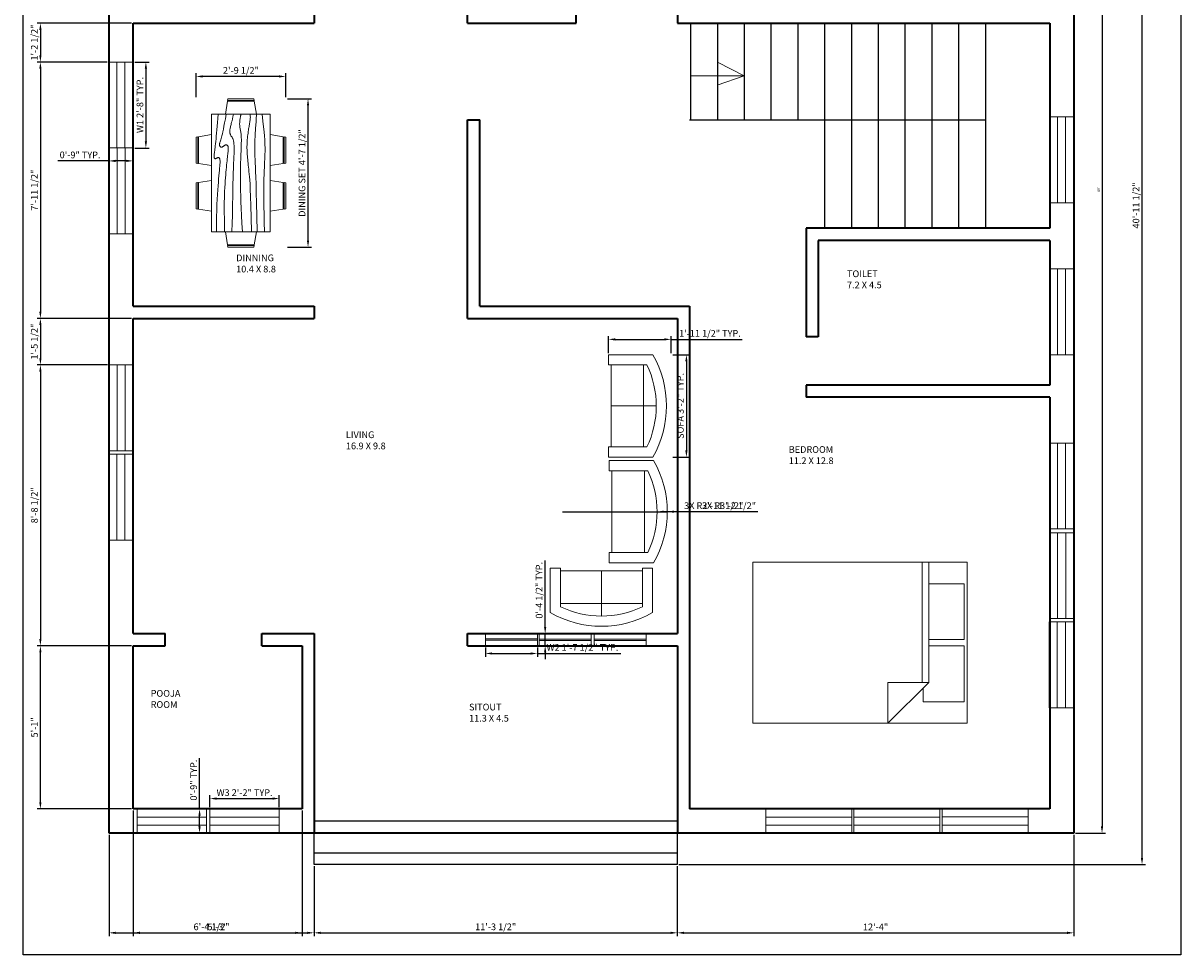
# Model space of a CAD drawing. Units: inches. Extents: x 185 to 617, y 27 to 601.
# Tile 1 of 2: x 185 to 617, y 27 to 374. Entities that reach past the tile are written whole.
import ezdxf

# ---------------------------------------------------------------- set-up
doc = ezdxf.new("R2010")
doc.units = ezdxf.units.IN
for name, color, linetype, lineweight in [('A-ANNO-DIMS', 2, 'Continuous', 18), ('A-ANNO-SYMB', 3, 'Continuous', 18), ('A-ANNO-TTLB', 7, 'Continuous', 25), ('A-AREA-IDEN', 7, 'Continuous', 18), ('A-FLOR-STRS', 7, 'Continuous', 25), ('A-FURN', 8, 'Continuous', 18), ('A-GLAZ', 4, 'Continuous', 18), ('A-WALL', 7, 'Continuous', 35)]:
    doc.layers.add(name, color=color, linetype=linetype, lineweight=lineweight)
doc.styles.get("Standard").update_dxf_attribs({"font": 'arial.ttf'})
doc.dimstyles.new('ISO-25', dxfattribs={"dimtxt": 2.5, "dimasz": 2.5, "dimexe": 1.25, "dimexo": 0.625, "dimtad": 1, "dimtxsty": 'Standard', "dimcen": 2.5, "dimadec": 0, "dimazin": 0, "dimtfac": 1, "dimtmove": 0, "dimatfit": 3, "dimfxl": 1, "dimarcsym": 0})

# ---------------------------------------------------------------- blocks, each defined once
blk = doc.blocks.new('Sofa - Roundback Loveseat 5 ft.')
for p, q in [((0, -32.44198), (0, -5.99998)), ((-24, -33.99998), (-24, -11.46958)), ((-23.9998, -13.38178), (23.99986, -13.38178)), ((24.00004, -33.99998), (24.00004, -11.46958)), ((-24, -32.44198), (24.00004, -32.44198))]:
    blk.add_line(p, q)
for points in [[(-24, -33.99998), (-30, -33.99998), (-30, -7.99998)], [(30.00004, -7.99998), (30.00004, -33.99998), (24.00004, -33.99998)]]:
    blk.add_lwpolyline(points)
for centre, radius, start, end in [((0, -60.24998), 60.24998, 60.13715, 119.8628), ((0, -61.38438), 55.38444, 64.32083, 115.6792)]:
    blk.add_arc(centre, radius, start, end)
blk = doc.blocks.new('Dining Set - 36 x 72 in.')
for p, q in [((-22.2343, 26.00059), (-23.4847, 17.99762)), ((-22.2304, 26), (-5.7608, 26)), ((-22, 27.5), (-22.1562, 26.50042)), ((-5.8416, 26.5), (-22.1534, 26.5)), ((-22, 27.5), (-6, 27.5)), ((-5.8437, 26.49966), (-6, 27.5)), ((-4.5152, 17.99762), (-5.7655, 25.99926)), ((5.7657, 26.00059), (4.5153, 17.99762)), ((5.7696, 26), (22.2392, 26)), ((6, 27.5), (5.8438, 26.50042)), ((22.1584, 26.5), (5.8466, 26.5)), ((6, 27.5), (22, 27.5)), ((22.1563, 26.49966), (22, 27.5)), ((23.4848, 17.99762), (22.2345, 25.99926)), ((36, 18), (-36, 18)), ((-36, 18), (-36, -18)), ((36, -18), (36, 18)), ((-45.5, 8), (-44.5004, 8.15617)), ((-45.5, 8), (-45.5, -8)), ((-44.5, -8.15843), (-44.5, 8.15338)), ((-44.0006, 8.23428), (-35.9976, 9.48474)), ((-44, 8.23041), (-44, -8.23915)), ((44.0006, 8.23428), (35.9976, 9.48474)), ((44, 8.23041), (44, -8.23915)), ((44.5, -8.15843), (44.5, 8.15338)), ((45.5, 8), (44.5005, 8.15617)), ((45.5, 8), (45.5, -8)), ((-44.4997, -8.15631), (-45.5, -8)), ((-35.9976, -9.48476), (-43.9993, -8.2345)), ((35.9976, -9.48476), (43.9993, -8.2345)), ((44.4997, -8.15631), (45.5, -8)), ((-36, -18), (36, -18)), ((-22.2343, -26.0006), (-23.4847, -17.99762)), ((-4.5152, -17.99762), (-5.7655, -25.99928)), ((5.7657, -26.0006), (4.5153, -17.99762)), ((23.4848, -17.99762), (22.2345, -25.99928)), ((-22.2304, -26), (-5.7608, -26)), ((-22, -27.5), (-22.1562, -26.50044)), ((-5.8416, -26.5), (-22.1534, -26.5)), ((-22, -27.5), (-6, -27.5)), ((-5.8437, -26.49967), (-6, -27.5)), ((5.7696, -26), (22.2392, -26)), ((6, -27.5), (5.8438, -26.50044)), ((22.1584, -26.5), (5.8466, -26.5)), ((6, -27.5), (22, -27.5)), ((22.1563, -26.49967), (22, -27.5))]:
    blk.add_line(p, q)
for points in [[(-36, 15), (-31.1772, 14.97754), (-26.8079, 14.91406), (-22.8538, 14.81543), (-19.276, 14.6875), (-16.0362, 14.53613), (-13.0957, 14.36718), (-10.4159, 14.18652), (-7.9583, 14), (-5.6904, 13.81315), (-3.6035, 13.63021), (-1.6954, 13.45508), (0.0365, 13.29166), (1.5945, 13.14388), (2.9811, 13.01562), (4.1988, 12.9108), (5.25, 12.83333), (6.1393, 12.78613), (6.8802, 12.76823), (7.4883, 12.77767), (7.9792, 12.8125), (8.3685, 12.87077), (8.6719, 12.95052), (8.9049, 13.0498), (9.0833, 13.16666), (9.2205, 13.29899), (9.3216, 13.44401), (9.3895, 13.59879), (9.4271, 13.76041), (9.4373, 13.92594), (9.4232, 14.09245), (9.3875, 14.257), (9.3333, 14.41666), (9.2638, 14.56917), (9.1836, 14.71484), (9.0975, 14.85465), (9.0104, 14.98958), (8.9272, 15.1206), (8.8529, 15.2487), (8.7922, 15.37483), (8.75, 15.5), (8.7305, 15.62467), (8.7344, 15.74739), (8.7617, 15.86621), (8.8125, 15.97916), (8.8867, 16.08431), (8.9844, 16.17968), (9.1055, 16.26334), (9.25, 16.33333), (9.4189, 16.38802), (9.6172, 16.42708), (9.8506, 16.45052), (10.125, 16.45833), (10.4463, 16.45052), (10.8203, 16.42708), (11.2529, 16.38802), (11.75, 16.33333), (12.3184, 16.26318), (12.9694, 16.17838), (13.7151, 16.07991), (14.5677, 15.96875), (15.5395, 15.84586), (16.6426, 15.71224), (17.8893, 15.56884), (19.2917, 15.41666), (20.859, 15.25667), (22.5879, 15.08984), (24.4721, 14.91715), (26.5052, 14.73958), (28.6809, 14.5581), (30.9929, 14.3737), (33.4347, 14.18733), (36, 14)], [(-36, 10), (-28.9766, 10.14274), (-23.1725, 10.20442), (-18.4241, 10.19775), (-14.5677, 10.13541), (-11.4399, 10.03011), (-8.877, 9.89453), (-6.7154, 9.74137), (-4.7917, 9.58333), (-2.9698, 9.43082), (-1.2246, 9.28515), (0.4415, 9.14534), (2.026, 9.01041), (3.5266, 8.87939), (4.9408, 8.7513), (6.266, 8.62516), (7.5, 8.5), (8.6411, 8.37549), (9.6914, 8.2539), (10.6538, 8.13818), (11.5312, 8.03125), (12.3267, 7.93603), (13.043, 7.85547), (13.6831, 7.79248), (14.25, 7.75), (14.7471, 7.7303), (15.1797, 7.73307), (15.5537, 7.75732), (15.875, 7.80208), (16.1494, 7.86637), (16.3828, 7.94922), (16.5811, 8.04964), (16.75, 8.16666), (16.8944, 8.29915), (17.0143, 8.44531), (17.1089, 8.60319), (17.1771, 8.77083), (17.218, 8.94629), (17.2305, 9.1276), (17.2137, 9.31282), (17.1667, 9.5), (17.0895, 9.6875), (16.987, 9.875), (16.8649, 10.0625), (16.7292, 10.25), (16.5856, 10.4375), (16.4401, 10.625), (16.2985, 10.8125), (16.1667, 11), (16.05, 11.18733), (15.9518, 11.3737), (15.8752, 11.5581), (15.8229, 11.73958), (15.798, 11.91715), (15.8034, 12.08984), (15.842, 12.25667), (15.9167, 12.41666), (16.0295, 12.56836), (16.1784, 12.70833), (16.3605, 12.83268), (16.5729, 12.9375), (16.8127, 13.01888), (17.0768, 13.07291), (17.3625, 13.0957), (17.6667, 13.08333), (17.9894, 13.03312), (18.3418, 12.94726), (18.7382, 12.82918), (19.1927, 12.68229), (19.7195, 12.51001), (20.3327, 12.31575), (21.0465, 12.10294), (21.875, 11.875), (22.8357, 11.63354), (23.959, 11.37304), (25.2786, 11.08618), (26.8282, 10.76562), (28.6414, 10.40405), (30.752, 9.99414), (33.1936, 9.52856), (36, 9)], [(-36, 5.5), (-30.7157, 5.3348), (-26.069, 5.20963), (-21.9946, 5.11767), (-18.4271, 5.05208), (-15.3009, 5.00602), (-12.5508, 4.97265), (-10.1112, 4.94515), (-7.9167, 4.91666), (-5.909, 4.88167), (-4.0586, 4.83984), (-2.3429, 4.79215), (-0.7396, 4.73958), (0.7739, 4.6831), (2.22, 4.6237), (3.6213, 4.56233), (5, 4.5), (6.373, 4.43782), (7.7344, 4.3776), (9.0723, 4.32129), (10.375, 4.27083), (11.6309, 4.22819), (12.8281, 4.19531), (13.9551, 4.17415), (15, 4.16666), (15.954, 4.17448), (16.819, 4.19791), (17.6001, 4.23698), (18.3021, 4.29166), (18.9299, 4.36198), (19.4883, 4.44791), (19.9823, 4.54948), (20.4167, 4.66666), (20.7969, 4.79899), (21.1302, 4.94401), (21.4245, 5.09879), (21.6875, 5.26041), (21.9271, 5.42594), (22.1511, 5.59245), (22.3672, 5.757), (22.5834, 5.91666), (22.8065, 6.06868), (23.0404, 6.21093), (23.2879, 6.34147), (23.5521, 6.45833), (23.8358, 6.55957), (24.142, 6.64323), (24.4735, 6.70735), (24.8334, 6.75), (25.2235, 6.76969), (25.642, 6.76692), (26.0858, 6.74267), (26.5521, 6.69791), (27.0379, 6.63362), (27.5404, 6.55078), (28.0565, 6.45036), (28.5834, 6.33333), (29.1242, 6.19987), (29.7071, 6.04687), (30.3661, 5.87044), (31.1354, 5.66666), (32.0493, 5.43164), (33.142, 5.16146), (34.4475, 4.85221), (36, 4.5)], [(-36, -1), (-30.7915, -0.6591), (-26.0195, -0.38216), (-21.6519, -0.16284), (-17.6563, 0.00521), (-14.0005, 0.12833), (-10.6523, 0.21289), (-7.5796, 0.26522), (-4.75, 0.29166), (-2.134, 0.29793), (0.2878, 0.28711), (2.5317, 0.26163), (4.6146, 0.22396), (6.5529, 0.17651), (8.3633, 0.12174), (10.0623, 0.06209), (11.6667, 0), (13.1899, -0.06201), (14.6341, -0.1211), (15.9982, -0.17432), (17.2813, -0.21875), (18.4823, -0.25147), (19.6003, -0.26953), (20.6343, -0.27002), (21.5834, -0.25), (22.4481, -0.20768), (23.2357, -0.14584), (23.9549, -0.06836), (24.6146, 0.02083), (25.2235, 0.11784), (25.7904, 0.21875), (26.3241, 0.31966), (26.8334, 0.41666), (27.3265, 0.50618), (27.8099, 0.58593), (28.2894, 0.65397), (28.7709, 0.70833), (29.2601, 0.74707), (29.763, 0.76823), (30.2855, 0.76985), (30.8334, 0.75), (31.4088, 0.70784), (31.9994, 0.64713), (32.589, 0.57275), (33.1615, 0.48958), (33.7008, 0.4025), (34.1908, 0.3164), (34.6153, 0.23616), (34.9584, 0.16666), (35.2099, 0.11165), (35.3848, 0.07031), (35.504, 0.04069), (35.5886, 0.02083), (35.6594, 0.00879), (35.7377, 0.0026), (35.8442, 0.00032), (36, 0)], [(-36, -6.5), (-27.1843, -6.31267), (-20.084, -6.1263), (-14.469, -5.9419), (-10.1094, -5.76042), (-6.7752, -5.58285), (-4.2363, -5.41016), (-2.2629, -5.24333), (-0.625, -5.08334), (0.8708, -4.93099), (2.2715, -4.78646), (3.5872, -4.64974), (4.8281, -4.52084), (6.0046, -4.39974), (7.127, -4.28646), (8.2053, -4.18099), (9.25, -4.08334), (10.2705, -3.99382), (11.2734, -3.91407), (12.2647, -3.84603), (13.25, -3.79167), (14.2354, -3.75293), (15.2266, -3.73177), (16.2295, -3.73015), (17.25, -3.75), (18.2912, -3.79248), (19.3451, -3.85547), (20.4009, -3.93604), (21.4479, -4.03125), (22.4754, -4.13819), (23.4727, -4.25391), (24.4289, -4.37549), (25.3334, -4.5), (26.1785, -4.62492), (26.9694, -4.74935), (27.7145, -4.87281), (28.4219, -4.99479), (29.1, -5.11483), (29.7572, -5.23242), (30.4016, -5.34709), (31.0417, -5.45834), (31.6837, -5.56437), (32.3262, -5.65821), (32.9658, -5.73153), (33.599, -5.77604), (34.2224, -5.78345), (34.8327, -5.74545), (35.4264, -5.65373), (36, -5.5)], [(-36, -10), (-26.4022, -9.81299), (-18.4675, -9.62891), (-11.9839, -9.45069), (-6.7396, -9.28125), (-2.5226, -9.12354), (0.8789, -8.98047), (3.6769, -8.85498), (6.0833, -8.75), (8.2767, -8.66765), (10.3021, -8.60677), (12.1712, -8.56543), (13.8958, -8.54167), (15.4876, -8.53353), (16.9583, -8.53907), (18.3197, -8.55632), (19.5834, -8.58334), (20.7616, -8.61841), (21.8685, -8.66081), (22.9188, -8.71004), (23.9271, -8.76563), (24.9081, -8.82707), (25.8763, -8.89388), (26.8465, -8.96558), (27.8334, -9.04167), (28.8474, -9.12118), (29.8828, -9.20117), (30.93, -9.27824), (31.9792, -9.34896), (33.0205, -9.40991), (34.0443, -9.45768), (35.0407, -9.48885), (36, -9.5)], [(-36, -14.5), (-30.0881, -14.33513), (-25.0332, -14.21224), (-20.7312, -14.12647), (-17.0781, -14.07292), (-13.97, -14.04671), (-11.3027, -14.04297), (-8.9724, -14.05681), (-6.875, -14.08334), (-4.9224, -14.11833), (-3.0905, -14.16016), (-1.3709, -14.20785), (0.2448, -14.26042), (1.7647, -14.3169), (3.1973, -14.3763), (4.5507, -14.43767), (5.8333, -14.5), (7.0554, -14.5621), (8.235, -14.62175), (9.3922, -14.67652), (10.5469, -14.72396), (11.7192, -14.76164), (12.929, -14.78711), (14.1965, -14.79794), (15.5417, -14.79167), (16.9933, -14.76424), (18.6152, -14.70508), (20.4804, -14.60197), (22.6615, -14.44271), (25.2312, -14.21509), (28.2624, -13.9069), (31.8277, -13.50594), (36, -13)]]:
    blk.add_lwpolyline(points)
blk = doc.blocks.new('Bed - Queen')
for p, q in [((0, -80.00003), (0, 0)), ((0, 0), (59.99999, 0)), ((59.99999, 0), (59.99999, -80.00003)), ((7.99999, -1.2), (28.79998, -1.2)), ((7.99999, -14.4), (7.99999, -1.2)), ((28.79998, -1.2), (28.79998, -14.4)), ((31.19999, -1.2), (51.99999, -1.2)), ((31.19999, -14.4), (31.19999, -1.2)), ((51.99999, -1.2), (51.99999, -16.4)), ((0, -14.4), (44.8, -14.4)), ((44.8, -16.8), (0, -16.8)), ((59.99999, -29.6), (44.8, -14.4)), ((44.8, -14.4), (44.8, -29.6)), ((51.99999, -16.4), (46.79936, -16.4)), ((44.8, -29.6), (59.99999, -29.6)), ((59.99999, -80.00003), (0, -80.00003))]:
    blk.add_line(p, q)
blk = doc.blocks.new('*D7')
at = {"layer": 'A-ANNO-DIMS', "color": 0, "lineweight": -2, "transparency": 16777216}
for p, q in [((577.73, 552.31), (588.89, 552.31)), ((587.64, 549.81), (587.64, 74.81)), ((577.73, 72.31), (588.89, 72.31))]:
    blk.add_line(p, q, dxfattribs=at)
at = {"layer": 'A-ANNO-DIMS', "color": 0, "transparency": 16777216}
for points in [[(587.22, 549.81), (588.05, 549.81), (587.64, 552.31)], [(587.22, 74.81), (588.05, 74.81), (587.64, 72.31)]]:
    blk.add_solid(points, dxfattribs=at)
at = {"layer": 'Defpoints', "color": 0, "transparency": 16777216}
for p in [(577.11, 552.31), (577.11, 72.31), (587.64, 72.31)]:
    blk.add_point(p, dxfattribs=at)
at = {"layer": 'A-ANNO-DIMS', "color": 0, "transparency": 16777216, "insert": (586.5, 312.31), "char_height": 1, "attachment_point": 5, "rotation": 90}
blk.add_mtext("40'", dxfattribs=at)
blk = doc.blocks.new('WIN-32IN-EXT')
for p, q in [((0, 0), (0, 32.06)), ((0, 32.06), (9, 32.06)), ((3, 32.06), (3, 0)), ((6, 0), (6, 32.06)), ((9, 32.06), (9, 0)), ((9, 0), (0, 0))]:
    blk.add_line(p, q)
blk = doc.blocks.new('WIN-19IN-SITOUT')
for p, q in [((0, 0), (0, 4.5)), ((0, 4.5), (19.38, 4.5)), ((19.38, 4.5), (19.38, 0)), ((0, 2.5), (19.38, 2.5)), ((19.38, 2), (0, 2)), ((19.38, 0), (0, 0))]:
    blk.add_line(p, q)
blk = doc.blocks.new('WIN-26IN-EXT')
for p, q in [((0, 0), (0, 9)), ((0, 9), (25.86, 9)), ((25.86, 9), (25.86, 0)), ((25.86, 6), (0, 6)), ((0, 3), (25.86, 3)), ((25.86, 0), (0, 0))]:
    blk.add_line(p, q)
blk = doc.blocks.new('*D11')
at = {"layer": 'A-ANNO-DIMS', "color": 0, "lineweight": -2, "transparency": 16777216}
for p, q in [((226.67, 359.92), (232.11, 359.92)), ((230.86, 357.42), (230.86, 330.35)), ((226.67, 327.85), (232.11, 327.85))]:
    blk.add_line(p, q, dxfattribs=at)
at = {"layer": 'A-ANNO-DIMS', "color": 0, "transparency": 16777216}
for points in [[(230.44, 357.42), (231.27, 357.42), (230.86, 359.92)], [(230.44, 330.35), (231.27, 330.35), (230.86, 327.85)]]:
    blk.add_solid(points, dxfattribs=at)
at = {"layer": 'Defpoints', "color": 0, "transparency": 16777216}
for p in [(226.05, 359.92), (226.05, 327.85), (230.86, 327.85)]:
    blk.add_point(p, dxfattribs=at)
at = {"layer": 'A-ANNO-DIMS', "color": 0, "transparency": 16777216, "insert": (228.96, 343.88), "char_height": 2.5, "attachment_point": 5, "rotation": 90}
blk.add_mtext('W1 2\'-8" TYP.', dxfattribs=at)
blk = doc.blocks.new('*D12')
at = {"layer": 'A-ANNO-DIMS', "color": 0, "lineweight": -2, "transparency": 16777216}
for p, q in [((217.05, 327.23), (217.05, 321.79)), ((226.05, 327.23), (226.05, 321.79)), ((217.05, 323.04), (198.06, 323.04)), ((223.55, 323.04), (219.55, 323.04))]:
    blk.add_line(p, q, dxfattribs=at)
at = {"layer": 'A-ANNO-DIMS', "color": 0, "transparency": 16777216}
for points in [[(219.55, 323.46), (219.55, 322.62), (217.05, 323.04)], [(223.55, 323.46), (223.55, 322.62), (226.05, 323.04)]]:
    blk.add_solid(points, dxfattribs=at)
at = {"layer": 'Defpoints', "color": 0, "transparency": 16777216}
for p in [(217.05, 327.85), (226.05, 327.85), (217.05, 323.04)]:
    blk.add_point(p, dxfattribs=at)
at = {"layer": 'A-ANNO-DIMS', "color": 0, "transparency": 16777216, "insert": (206.3, 324.94), "char_height": 2.5, "attachment_point": 5}
blk.add_mtext('0\'-9" TYP.', dxfattribs=at)
blk = doc.blocks.new('*D13')
at = {"layer": 'A-ANNO-DIMS', "color": 0, "lineweight": -2, "transparency": 16777216}
for p, q in [((357.55, 141.6), (357.55, 138.06)), ((360.05, 139.31), (374.43, 139.31)), ((376.93, 141.6), (376.93, 138.06)), ((376.93, 139.31), (408.06, 139.31))]:
    blk.add_line(p, q, dxfattribs=at)
at = {"layer": 'A-ANNO-DIMS', "color": 0, "transparency": 16777216}
for points in [[(360.05, 139.73), (360.05, 138.9), (357.55, 139.31)], [(374.43, 139.73), (374.43, 138.9), (376.93, 139.31)]]:
    blk.add_solid(points, dxfattribs=at)
at = {"layer": 'Defpoints', "color": 0, "transparency": 16777216}
for p in [(357.55, 142.22), (376.93, 142.22), (376.93, 139.31)]:
    blk.add_point(p, dxfattribs=at)
at = {"layer": 'A-ANNO-DIMS', "color": 0, "transparency": 16777216, "insert": (393.75, 141.23), "char_height": 2.5, "attachment_point": 5}
blk.add_mtext('W2 1\'-7 1/2" TYP.', dxfattribs=at)
blk = doc.blocks.new('*D14')
at = {"layer": 'A-ANNO-DIMS', "color": 0, "lineweight": -2, "transparency": 16777216}
for p, q in [((379.84, 149.22), (379.84, 174.04)), ((377.56, 146.72), (381.09, 146.72)), ((379.84, 142.22), (379.84, 146.72)), ((377.56, 142.22), (381.09, 142.22)), ((379.84, 139.72), (379.84, 137.22))]:
    blk.add_line(p, q, dxfattribs=at)
at = {"layer": 'A-ANNO-DIMS', "color": 0, "transparency": 16777216}
for points in [[(379.42, 149.22), (380.26, 149.22), (379.84, 146.72)], [(379.42, 139.72), (380.26, 139.72), (379.84, 142.22)]]:
    blk.add_solid(points, dxfattribs=at)
at = {"layer": 'Defpoints', "color": 0, "transparency": 16777216}
for p in [(376.93, 146.72), (379.84, 146.72), (376.93, 142.22)]:
    blk.add_point(p, dxfattribs=at)
at = {"layer": 'A-ANNO-DIMS', "color": 0, "transparency": 16777216, "insert": (377.92, 162.88), "char_height": 2.5, "attachment_point": 5, "rotation": 90}
blk.add_mtext('0\'-4 1/2" TYP.', dxfattribs=at)
blk = doc.blocks.new('*D15')
at = {"layer": 'A-ANNO-DIMS', "color": 0, "lineweight": -2, "transparency": 16777216}
for p, q in [((254.75, 81.95), (254.75, 86.45)), ((280.61, 81.95), (280.61, 86.45)), ((257.25, 85.2), (278.11, 85.2))]:
    blk.add_line(p, q, dxfattribs=at)
at = {"layer": 'A-ANNO-DIMS', "color": 0, "transparency": 16777216}
for points in [[(257.25, 85.62), (257.25, 84.78), (254.75, 85.2)], [(278.11, 85.62), (278.11, 84.78), (280.61, 85.2)]]:
    blk.add_solid(points, dxfattribs=at)
at = {"layer": 'Defpoints', "color": 0, "transparency": 16777216}
for p in [(280.61, 85.2), (254.75, 81.32), (280.61, 81.32)]:
    blk.add_point(p, dxfattribs=at)
at = {"layer": 'A-ANNO-DIMS', "color": 0, "transparency": 16777216, "insert": (267.68, 87.1), "char_height": 2.5, "attachment_point": 5}
blk.add_mtext('W3 2\'-2" TYP.', dxfattribs=at)
blk = doc.blocks.new('*D16')
at = {"layer": 'A-ANNO-DIMS', "color": 0, "lineweight": -2, "transparency": 16777216}
for p, q in [((250.88, 81.32), (250.88, 100.31)), ((254.13, 81.32), (249.63, 81.32)), ((250.88, 74.82), (250.88, 78.82)), ((254.13, 72.32), (249.63, 72.32))]:
    blk.add_line(p, q, dxfattribs=at)
at = {"layer": 'A-ANNO-DIMS', "color": 0, "transparency": 16777216}
for points in [[(250.46, 78.82), (251.29, 78.82), (250.88, 81.32)], [(250.46, 74.82), (251.29, 74.82), (250.88, 72.32)]]:
    blk.add_solid(points, dxfattribs=at)
at = {"layer": 'Defpoints', "color": 0, "transparency": 16777216}
for p in [(250.88, 81.32), (254.75, 81.32), (254.75, 72.32)]:
    blk.add_point(p, dxfattribs=at)
at = {"layer": 'A-ANNO-DIMS', "color": 0, "transparency": 16777216, "insert": (248.97, 92.07), "char_height": 2.5, "attachment_point": 5, "rotation": 90}
blk.add_mtext('0\'-9" TYP.', dxfattribs=at)
blk = doc.blocks.new('*D17')
at = {"layer": 'A-ANNO-DIMS', "color": 0, "lineweight": -2, "transparency": 16777216}
for p, q in [((427.44, 250.74), (433.8, 250.74)), ((432.55, 248.24), (432.55, 215.03)), ((427.44, 212.53), (433.8, 212.53))]:
    blk.add_line(p, q, dxfattribs=at)
at = {"layer": 'A-ANNO-DIMS', "color": 0, "transparency": 16777216}
for points in [[(432.13, 248.24), (432.96, 248.24), (432.55, 250.74)], [(432.13, 215.03), (432.96, 215.03), (432.55, 212.53)]]:
    blk.add_solid(points, dxfattribs=at)
at = {"layer": 'Defpoints', "color": 0, "transparency": 16777216}
for p in [(426.82, 250.74), (426.82, 212.53), (432.55, 212.53)]:
    blk.add_point(p, dxfattribs=at)
at = {"layer": 'A-ANNO-DIMS', "color": 0, "transparency": 16777216, "insert": (430.63, 231.64), "char_height": 2.5, "attachment_point": 5, "rotation": 90}
blk.add_mtext('SOFA 3\'-2" TYP.', dxfattribs=at)
blk = doc.blocks.new('*D18')
at = {"layer": 'A-ANNO-DIMS', "color": 0, "lineweight": -2, "transparency": 16777216}
for p, q in [((403.47, 251.36), (403.47, 257.72)), ((405.97, 256.47), (424.32, 256.47)), ((426.82, 251.36), (426.82, 257.72)), ((426.82, 256.47), (453.34, 256.47))]:
    blk.add_line(p, q, dxfattribs=at)
at = {"layer": 'A-ANNO-DIMS', "color": 0, "transparency": 16777216}
for points in [[(405.97, 256.88), (405.97, 256.05), (403.47, 256.47)], [(424.32, 256.88), (424.32, 256.05), (426.82, 256.47)]]:
    blk.add_solid(points, dxfattribs=at)
at = {"layer": 'Defpoints', "color": 0, "transparency": 16777216}
for p in [(426.82, 256.47), (403.47, 250.74), (426.82, 250.74)]:
    blk.add_point(p, dxfattribs=at)
at = {"layer": 'A-ANNO-DIMS', "color": 0, "transparency": 16777216, "insert": (441.33, 258.38), "char_height": 2.5, "attachment_point": 5}
blk.add_mtext('1\'-11 1/2" TYP.', dxfattribs=at)
blk = doc.blocks.new('*D21')
at = {"layer": 'A-ANNO-DIMS', "color": 0, "lineweight": -2, "transparency": 16777216}
for p, q in [((283.68, 346.23), (292.61, 346.23)), ((291.36, 293.33), (291.36, 343.73)), ((283.68, 290.83), (292.61, 290.83))]:
    blk.add_line(p, q, dxfattribs=at)
at = {"layer": 'A-ANNO-DIMS', "color": 0, "transparency": 16777216}
for points in [[(290.95, 343.73), (291.78, 343.73), (291.36, 346.23)], [(290.95, 293.33), (291.78, 293.33), (291.36, 290.83)]]:
    blk.add_solid(points, dxfattribs=at)
at = {"layer": 'Defpoints', "color": 0, "transparency": 16777216}
for p in [(283.05, 346.23), (291.36, 346.23), (283.05, 290.83)]:
    blk.add_point(p, dxfattribs=at)
at = {"layer": 'A-ANNO-DIMS', "color": 0, "transparency": 16777216, "insert": (289.44, 318.53), "char_height": 2.5, "attachment_point": 5, "rotation": 90}
blk.add_mtext('DINING SET 4\'-7 1/2"', dxfattribs=at)
blk = doc.blocks.new('*D22')
at = {"layer": 'A-ANNO-DIMS', "color": 0, "lineweight": -2, "transparency": 16777216}
for p, q in [((249.57, 346.85), (249.57, 355.79)), ((280.55, 354.54), (252.07, 354.54)), ((283.05, 346.85), (283.05, 355.79))]:
    blk.add_line(p, q, dxfattribs=at)
at = {"layer": 'A-ANNO-DIMS', "color": 0, "transparency": 16777216}
for points in [[(252.07, 354.95), (252.07, 354.12), (249.57, 354.54)], [(280.55, 354.95), (280.55, 354.12), (283.05, 354.54)]]:
    blk.add_solid(points, dxfattribs=at)
at = {"layer": 'Defpoints', "color": 0, "transparency": 16777216}
for p in [(249.57, 354.54), (249.57, 346.23), (283.05, 346.23)]:
    blk.add_point(p, dxfattribs=at)
at = {"layer": 'A-ANNO-DIMS', "color": 0, "transparency": 16777216, "insert": (266.31, 356.46), "char_height": 2.5, "attachment_point": 5}
blk.add_mtext('2\'-9 1/2"', dxfattribs=at)
blk = doc.blocks.new('*D25')
at = {"layer": 'A-ANNO-DIMS', "color": 0, "lineweight": -2, "transparency": 16777216}
for p, q in [((577.73, 552.31), (603.81, 552.31)), ((602.56, 63.07), (602.56, 549.81)), ((429.78, 60.57), (603.81, 60.57))]:
    blk.add_line(p, q, dxfattribs=at)
at = {"layer": 'A-ANNO-DIMS', "color": 0, "transparency": 16777216}
for points in [[(602.14, 549.81), (602.97, 549.81), (602.56, 552.31)], [(602.14, 63.07), (602.97, 63.07), (602.56, 60.57)]]:
    blk.add_solid(points, dxfattribs=at)
at = {"layer": 'Defpoints', "color": 0, "transparency": 16777216}
for p in [(577.11, 552.31), (602.56, 552.31), (429.16, 60.57)]:
    blk.add_point(p, dxfattribs=at)
at = {"layer": 'A-ANNO-DIMS', "color": 0, "transparency": 16777216, "insert": (600.64, 306.44), "char_height": 2.5, "attachment_point": 5, "rotation": 90}
blk.add_mtext('40\'-11 1/2"', dxfattribs=at)
blk = doc.blocks.new('*D26')
at = {"layer": 'A-ANNO-DIMS', "color": 0, "lineweight": -2, "transparency": 16777216}
for p, q in [((226.11, 80.69), (226.11, 33.87)), ((289.11, 80.69), (289.11, 33.87)), ((228.61, 35.12), (286.61, 35.12))]:
    blk.add_line(p, q, dxfattribs=at)
at = {"layer": 'A-ANNO-DIMS', "color": 0, "transparency": 16777216}
for points in [[(228.61, 35.54), (228.61, 34.7), (226.11, 35.12)], [(286.61, 35.54), (286.61, 34.7), (289.11, 35.12)]]:
    blk.add_solid(points, dxfattribs=at)
at = {"layer": 'Defpoints', "color": 0, "transparency": 16777216}
for p in [(226.11, 81.31), (289.11, 81.31), (289.11, 35.12)]:
    blk.add_point(p, dxfattribs=at)
at = {"layer": 'A-ANNO-DIMS', "color": 0, "transparency": 16777216, "insert": (257.61, 37.02), "char_height": 2.5, "attachment_point": 5}
blk.add_mtext('5\'-3"', dxfattribs=at)
blk = doc.blocks.new('*D27')
at = {"layer": 'A-ANNO-DIMS', "color": 0, "lineweight": -2, "transparency": 16777216}
for p, q in [((225.48, 142.21), (190.25, 142.21)), ((191.5, 83.81), (191.5, 139.71)), ((225.48, 81.31), (190.25, 81.31))]:
    blk.add_line(p, q, dxfattribs=at)
at = {"layer": 'A-ANNO-DIMS', "color": 0, "transparency": 16777216}
for points in [[(191.08, 139.71), (191.91, 139.71), (191.5, 142.21)], [(191.08, 83.81), (191.91, 83.81), (191.5, 81.31)]]:
    blk.add_solid(points, dxfattribs=at)
at = {"layer": 'Defpoints', "color": 0, "transparency": 16777216}
for p in [(191.5, 142.21), (226.11, 142.21), (226.11, 81.31)]:
    blk.add_point(p, dxfattribs=at)
at = {"layer": 'A-ANNO-DIMS', "color": 0, "transparency": 16777216, "insert": (189.6, 111.76), "char_height": 2.5, "attachment_point": 5, "rotation": 90}
blk.add_mtext('5\'-1"', dxfattribs=at)
blk = doc.blocks.new('*D28')
at = {"layer": 'A-ANNO-DIMS', "color": 0, "lineweight": -2, "transparency": 16777216}
for p, q in [((217.11, 71.69), (217.11, 33.87)), ((293.59, 59.94), (293.59, 33.87)), ((219.61, 35.12), (291.09, 35.12))]:
    blk.add_line(p, q, dxfattribs=at)
at = {"layer": 'A-ANNO-DIMS', "color": 0, "transparency": 16777216}
for points in [[(219.61, 35.54), (219.61, 34.7), (217.11, 35.12)], [(291.09, 35.54), (291.09, 34.7), (293.59, 35.12)]]:
    blk.add_solid(points, dxfattribs=at)
at = {"layer": 'Defpoints', "color": 0, "transparency": 16777216}
for p in [(217.11, 72.31), (293.59, 60.57), (293.59, 35.12)]:
    blk.add_point(p, dxfattribs=at)
at = {"layer": 'A-ANNO-DIMS', "color": 0, "transparency": 16777216, "insert": (255.35, 37.04), "char_height": 2.5, "attachment_point": 5}
blk.add_mtext('6\'-4 1/2"', dxfattribs=at)
blk = doc.blocks.new('*D29')
at = {"layer": 'A-ANNO-DIMS', "color": 0, "lineweight": -2, "transparency": 16777216}
for p, q in [((293.59, 59.94), (293.59, 33.87)), ((429.16, 59.94), (429.16, 33.87)), ((296.09, 35.12), (426.66, 35.12))]:
    blk.add_line(p, q, dxfattribs=at)
at = {"layer": 'A-ANNO-DIMS', "color": 0, "transparency": 16777216}
for points in [[(296.09, 35.54), (296.09, 34.7), (293.59, 35.12)], [(426.66, 35.54), (426.66, 34.7), (429.16, 35.12)]]:
    blk.add_solid(points, dxfattribs=at)
at = {"layer": 'Defpoints', "color": 0, "transparency": 16777216}
for p in [(293.59, 60.57), (429.16, 60.57), (429.16, 35.12)]:
    blk.add_point(p, dxfattribs=at)
at = {"layer": 'A-ANNO-DIMS', "color": 0, "transparency": 16777216, "insert": (361.38, 37.04), "char_height": 2.5, "attachment_point": 5}
blk.add_mtext('11\'-3 1/2"', dxfattribs=at)
blk = doc.blocks.new('*D30')
at = {"layer": 'A-ANNO-DIMS', "color": 0, "lineweight": -2, "transparency": 16777216}
for p, q in [((577.11, 71.69), (577.11, 33.87)), ((429.16, 59.94), (429.16, 33.87)), ((431.66, 35.12), (574.61, 35.12))]:
    blk.add_line(p, q, dxfattribs=at)
at = {"layer": 'A-ANNO-DIMS', "color": 0, "transparency": 16777216}
for points in [[(431.66, 35.54), (431.66, 34.7), (429.16, 35.12)], [(574.61, 35.54), (574.61, 34.7), (577.11, 35.12)]]:
    blk.add_solid(points, dxfattribs=at)
at = {"layer": 'Defpoints', "color": 0, "transparency": 16777216}
for p in [(577.11, 72.31), (429.16, 60.57), (577.11, 35.12)]:
    blk.add_point(p, dxfattribs=at)
at = {"layer": 'A-ANNO-DIMS', "color": 0, "transparency": 16777216, "insert": (503.13, 37), "char_height": 2.5, "attachment_point": 5}
blk.add_mtext('12\'-4"', dxfattribs=at)
blk = doc.blocks.new('*D40')
at = {"layer": 'A-ANNO-DIMS', "color": 0, "lineweight": -2, "transparency": 16777216}
for p, q in [((225.48, 374.41), (190.25, 374.41)), ((191.5, 371.91), (191.5, 362.42)), ((216.42, 359.92), (190.25, 359.92))]:
    blk.add_line(p, q, dxfattribs=at)
at = {"layer": 'A-ANNO-DIMS', "color": 0, "transparency": 16777216}
for points in [[(191.08, 371.91), (191.91, 371.91), (191.5, 374.41)], [(191.08, 362.42), (191.91, 362.42), (191.5, 359.92)]]:
    blk.add_solid(points, dxfattribs=at)
at = {"layer": 'Defpoints', "color": 0, "transparency": 16777216}
for p in [(226.11, 374.41), (191.5, 359.92), (217.05, 359.92)]:
    blk.add_point(p, dxfattribs=at)
at = {"layer": 'A-ANNO-DIMS', "color": 0, "transparency": 16777216, "insert": (189.58, 367.17), "char_height": 2.5, "attachment_point": 5, "rotation": 90}
blk.add_mtext('1\'-2 1/2"', dxfattribs=at)
blk = doc.blocks.new('*D41')
at = {"layer": 'A-ANNO-DIMS', "color": 0, "lineweight": -2, "transparency": 16777216}
for p, q in [((216.42, 359.92), (190.25, 359.92)), ((191.5, 357.42), (191.5, 266.81)), ((225.48, 264.31), (190.25, 264.31))]:
    blk.add_line(p, q, dxfattribs=at)
at = {"layer": 'A-ANNO-DIMS', "color": 0, "transparency": 16777216}
for points in [[(191.08, 357.42), (191.91, 357.42), (191.5, 359.92)], [(191.08, 266.81), (191.91, 266.81), (191.5, 264.31)]]:
    blk.add_solid(points, dxfattribs=at)
at = {"layer": 'Defpoints', "color": 0, "transparency": 16777216}
for p in [(217.05, 359.92), (191.5, 264.31), (226.11, 264.31)]:
    blk.add_point(p, dxfattribs=at)
at = {"layer": 'A-ANNO-DIMS', "color": 0, "transparency": 16777216, "insert": (189.58, 312.12), "char_height": 2.5, "attachment_point": 5, "rotation": 90}
blk.add_mtext('7\'-11 1/2"', dxfattribs=at)
blk = doc.blocks.new('*D42')
at = {"layer": 'A-ANNO-DIMS', "color": 0, "lineweight": -2, "transparency": 16777216}
for p, q in [((225.48, 264.31), (190.25, 264.31)), ((191.5, 261.81), (191.5, 249.45)), ((216.49, 246.95), (190.25, 246.95))]:
    blk.add_line(p, q, dxfattribs=at)
at = {"layer": 'A-ANNO-DIMS', "color": 0, "transparency": 16777216}
for points in [[(191.08, 261.81), (191.91, 261.81), (191.5, 264.31)], [(191.08, 249.45), (191.91, 249.45), (191.5, 246.95)]]:
    blk.add_solid(points, dxfattribs=at)
at = {"layer": 'Defpoints', "color": 0, "transparency": 16777216}
for p in [(226.11, 264.31), (191.5, 246.95), (217.11, 246.95)]:
    blk.add_point(p, dxfattribs=at)
at = {"layer": 'A-ANNO-DIMS', "color": 0, "transparency": 16777216, "insert": (189.58, 255.63), "char_height": 2.5, "attachment_point": 5, "rotation": 90}
blk.add_mtext('1\'-5 1/2"', dxfattribs=at)
blk = doc.blocks.new('*D43')
at = {"layer": 'A-ANNO-DIMS', "color": 0, "lineweight": -2, "transparency": 16777216}
for p, q in [((216.49, 246.95), (190.25, 246.95)), ((191.5, 244.45), (191.5, 144.71)), ((225.48, 142.21), (190.25, 142.21))]:
    blk.add_line(p, q, dxfattribs=at)
at = {"layer": 'A-ANNO-DIMS', "color": 0, "transparency": 16777216}
for points in [[(191.08, 244.45), (191.91, 244.45), (191.5, 246.95)], [(191.08, 144.71), (191.91, 144.71), (191.5, 142.21)]]:
    blk.add_solid(points, dxfattribs=at)
at = {"layer": 'Defpoints', "color": 0, "transparency": 16777216}
for p in [(217.11, 246.95), (191.5, 142.21), (226.11, 142.21)]:
    blk.add_point(p, dxfattribs=at)
at = {"layer": 'A-ANNO-DIMS', "color": 0, "transparency": 16777216, "insert": (189.58, 194.58), "char_height": 2.5, "attachment_point": 5, "rotation": 90}
blk.add_mtext('8\'-8 1/2"', dxfattribs=at)
blk = doc.blocks.new('*D46')
at = {"layer": 'A-ANNO-DIMS', "color": 0, "lineweight": -2, "transparency": 16777216}
for p, q in [((387.06, 192.2), (425.42, 192.2)), ((459.17, 192.2), (427.92, 192.2))]:
    blk.add_line(p, q, dxfattribs=at)
at = {"layer": 'A-ANNO-DIMS', "color": 0, "transparency": 16777216}
blk.add_solid([(427.92, 192.62), (427.92, 191.78), (425.42, 192.2)], dxfattribs=at)
at = {"layer": 'Defpoints', "color": 0, "transparency": 16777216}
for p in [(387.06, 192.2), (425.42, 192.2)]:
    blk.add_point(p, dxfattribs=at)
at = {"layer": 'A-ANNO-DIMS', "color": 0, "transparency": 16777216, "insert": (448.43, 194.12), "char_height": 2.5, "attachment_point": 5, "rotation": 0.0007}
blk.add_mtext('3X R3\'-2 1/2"', dxfattribs=at)
blk = doc.blocks.new('*D47')
at = {"layer": 'A-ANNO-DIMS', "color": 0, "lineweight": -2, "transparency": 16777216}
for p, q in [((386.33, 192.2), (421.6, 192.2)), ((454.47, 192.2), (424.1, 192.2))]:
    blk.add_line(p, q, dxfattribs=at)
at = {"layer": 'A-ANNO-DIMS', "color": 0, "transparency": 16777216}
blk.add_solid([(424.1, 192.62), (424.1, 191.78), (421.6, 192.2)], dxfattribs=at)
at = {"layer": 'Defpoints', "color": 0, "transparency": 16777216}
for p in [(386.33, 192.2), (421.6, 192.2)]:
    blk.add_point(p, dxfattribs=at)
at = {"layer": 'A-ANNO-DIMS', "color": 0, "transparency": 16777216, "insert": (442.75, 194.12), "char_height": 2.5, "attachment_point": 5, "rotation": 0.0007}
blk.add_mtext('3X R2\'-11 1/2"', dxfattribs=at)

msp = doc.modelspace()

# ---------------------------------------------------------------- linework, layer by layer
at = {"layer": 'A-ANNO-SYMB'}
for p, q in [((454.09, 354.81), (444.13, 359.92)), ((434.16, 354.81), (448.12, 354.81)), ((454.06, 354.8), (444.08, 351.26)), ((448.12, 354.81), (454.09, 354.81))]:
    msp.add_line(p, q, dxfattribs=at)
at = {"layer": 'A-ANNO-TTLB'}
msp.add_lwpolyline([(185.06, 600.8), (617.05, 600.8), (617.05, 26.91), (185.06, 26.91)], close=True, dxfattribs=at)
at = {"layer": 'A-FLOR-STRS'}
for p, q in [((434.11, 374.41), (434.11, 338.41)), ((444.11, 374.41), (444.11, 338.41)), ((454.11, 374.41), (454.11, 338.41)), ((464.11, 374.41), (464.11, 338.41)), ((474.11, 374.41), (474.11, 338.41)), ((484.11, 374.41), (484.11, 297.91)), ((494.11, 374.41), (494.11, 297.91)), ((504.11, 374.41), (504.11, 297.91)), ((514.11, 374.41), (514.11, 297.91)), ((524.11, 374.41), (524.11, 297.91)), ((534.11, 374.41), (534.11, 297.91)), ((544.11, 374.41), (544.11, 297.91)), ((433.71, 338.41), (544.11, 338.41)), ((429.21, 76.81), (293.61, 76.81)), ((429.21, 64.81), (293.61, 64.81))]:
    msp.add_line(p, q, dxfattribs=at)
msp.add_lwpolyline([(293.59, 72.3), (429.16, 72.3), (429.16, 60.57), (293.59, 60.57)], close=True, dxfattribs=at)
at = {"layer": 'A-WALL'}
for p, q in [((217.11, 72.31), (217.11, 552.31)), ((577.11, 552.31), (577.11, 72.31)), ((350.91, 374.41), (350.91, 543.31)), ((350.91, 374.41), (350.91, 543.31)), ((293.61, 378.91), (293.61, 374.41)), ((391.41, 374.41), (391.41, 378.91)), ((429.21, 378.91), (429.21, 374.41)), ((226.11, 374.41), (293.61, 374.41)), ((226.11, 268.81), (226.11, 374.41)), ((350.91, 374.41), (391.41, 374.41)), ((429.21, 374.41), (433.71, 374.41)), ((433.71, 374.41), (568.11, 374.41)), ((568.11, 374.41), (568.11, 297.91)), ((350.91, 338.41), (355.41, 338.41)), ((350.91, 264.31), (350.91, 338.41)), ((350.91, 264.31), (350.91, 338.41)), ((355.41, 268.81), (355.41, 338.41)), ((568.11, 297.91), (477.21, 297.91)), ((477.21, 297.91), (477.21, 257.41)), ((568.11, 293.41), (481.71, 293.41)), ((481.71, 293.41), (481.71, 257.41)), ((568.11, 293.41), (568.11, 239.41)), ((226.11, 268.81), (293.61, 268.81)), ((289.11, 268.81), (293.61, 268.81)), ((293.61, 268.81), (293.61, 264.31)), ((355.41, 268.81), (433.71, 268.81)), ((433.71, 268.81), (433.71, 81.31)), ((226.11, 264.31), (293.61, 264.31)), ((226.11, 146.71), (226.11, 264.31)), ((350.91, 264.31), (355.41, 264.31)), ((350.91, 264.31), (429.21, 264.31)), ((429.21, 264.31), (429.21, 146.71)), ((481.71, 257.41), (477.21, 257.41)), ((568.11, 239.41), (477.21, 239.41)), ((568.11, 239.41), (477.21, 239.41)), ((477.21, 239.41), (477.21, 234.91)), ((568.11, 234.91), (477.21, 234.91)), ((568.11, 234.91), (477.21, 234.91)), ((568.11, 234.91), (568.11, 81.31)), ((226.11, 146.71), (238.11, 146.71)), ((238.11, 142.21), (238.11, 146.71)), ((274.11, 142.21), (274.11, 146.71)), ((274.11, 146.71), (293.61, 146.71)), ((293.61, 146.71), (293.61, 72.31)), ((350.91, 142.21), (350.91, 146.71)), ((350.91, 142.21), (350.91, 146.71)), ((350.91, 146.71), (429.21, 146.71)), ((226.11, 81.31), (226.11, 142.21)), ((226.11, 142.21), (238.11, 142.21)), ((274.11, 142.21), (289.11, 142.21)), ((289.11, 142.21), (289.11, 81.31)), ((350.91, 142.21), (429.21, 142.21)), ((429.21, 142.21), (429.21, 72.31)), ((289.11, 81.31), (226.11, 81.31)), ((568.11, 81.31), (433.71, 81.31)), ((577.11, 72.31), (217.11, 72.31))]:
    msp.add_line(p, q, dxfattribs=at)

# ---------------------------------------------------------------- block references
at = {"layer": 'A-FURN'}
for name, p, xscale, yscale, zscale, rotation in [('Dining Set - 36 x 72 in.', (266.31, 318.53), 0.6087281652256751, 0.6087281652256751, 0.6087281652256751, 90), ('Sofa - Roundback Loveseat 5 ft.', (425.12, 231.64), 0.636694679750679, 0.636694679750679, 0.636694679750679, 270), ('Sofa - Roundback Loveseat 5 ft.', (425.42, 192.2), 0.636694679750679, 0.636694679750679, 0.636694679750679, 270), ('Sofa - Roundback Loveseat 5 ft.', (400.85, 149.47), 0.636694679750679, 0.636694679750679, 0.636694679750679, 180)]:
    msp.add_blockref(name, p, dxfattribs=dict(at, xscale=xscale, yscale=yscale, zscale=zscale, rotation=rotation))
at = {"layer": 'A-FURN', "rotation": 270}
msp.add_blockref('Bed - Queen', (537.35, 173.33), dxfattribs=at)
at = {"layer": 'A-GLAZ'}
for p, rotation in [((226.05, 359.92), 180), ((577.03, 339.49), 180), ((226.15, 327.9), 180), ((577, 282.73), 180), ((226.11, 246.95), 180), ((576.99, 217.82), 180), ((226.03, 213.6), 180), ((577.07, 184.37), 180), ((576.95, 151.13), 180), ((462.19, 81.22), 270.0000000000001), ((495.07, 81.29), 270.0000000000001), ((528, 81.34), 270.0000000000001)]:
    msp.add_blockref('WIN-32IN-EXT', p, dxfattribs=dict(at, rotation=rotation))
for name, p in [('WIN-19IN-SITOUT', (357.55, 142.22)), ('WIN-19IN-SITOUT', (377.61, 142.18)), ('WIN-19IN-SITOUT', (398.1, 142.16)), ('WIN-26IN-EXT', (227.59, 72.3)), ('WIN-26IN-EXT', (254.75, 72.32))]:
    msp.add_blockref(name, p, dxfattribs=at)

# ---------------------------------------------------------------- texts
at = {"layer": 'A-AREA-IDEN', "char_height": 2.5, "attachment_point": 1}
for s, width, insert in [('DINNING\\P10.4 X 8.8', 24.2796, (264.54, 288.12)), ('TOILET\\P7.2 X 4.5', 46.2477, (492.47, 282.19)), ('LIVING\\P16.9 X 9.8', 65.7836, (305.49, 222.15)), ('BEDROOM\\P11.2 X 12.8', 70.9213, (470.73, 216.64)), ('POOJA\\PROOM', 33.17, (232.64, 125.68)), ('SITOUT\\P11.3 X 4.5', 47.5205, (351.44, 120.57))]:
    msp.add_mtext_dynamic_manual_height_columns(s, width=width, gutter_width=12.5, heights=[0], dxfattribs=dict(at, insert=insert))

# ---------------------------------------------------------------- dimensions: what is measured, and where the dimension line sits
at = {"layer": 'A-ANNO-DIMS'}
for base, p1, p2, angle, override, picture, middle in [((602.56, 552.31), (429.16, 60.57), (577.11, 552.31), 90, {"dimdec": 1, "dimlfac": 1, "dimrnd": 0, "dimzin": 1, "dimdsep": 46, "dimlunit": 4, "dimfrac": 2}, '*D25', (600.64, 306.44)), ((587.64, 72.31), (577.11, 552.31), (577.11, 72.31), 90, {"dimtxt": 1, "dimdec": 0, "dimlunit": 3, "dimclrd": 0, "dimclre": 0, "dimclrt": 0, "dimtdec": 0}, '*D7', (586.5, 312.31)), ((191.5, 359.92), (226.11, 374.41), (217.05, 359.92), 90, {"dimdec": 1, "dimlfac": 1, "dimrnd": 0, "dimzin": 1, "dimdsep": 46, "dimlunit": 4, "dimfrac": 2}, '*D40', (189.58, 367.17)), ((191.5, 264.31), (217.05, 359.92), (226.11, 264.31), 90, {"dimdec": 1, "dimlfac": 1, "dimrnd": 0, "dimzin": 1, "dimdsep": 46, "dimlunit": 4, "dimfrac": 2}, '*D41', (189.58, 312.12)), ((249.57, 354.54), (283.05, 346.23), (249.57, 346.23), 180, {"dimdec": 1, "dimlfac": 1, "dimrnd": 0, "dimzin": 1, "dimdsep": 46, "dimlunit": 4, "dimfrac": 2}, '*D22', (266.31, 356.46)), ((191.5, 246.95), (226.11, 264.31), (217.11, 246.95), 90, {"dimdec": 1, "dimlfac": 1, "dimrnd": 0, "dimzin": 1, "dimdsep": 46, "dimlunit": 4, "dimfrac": 2}, '*D42', (189.58, 255.63)), ((191.5, 142.21), (217.11, 246.95), (226.11, 142.21), 90, {"dimdec": 1, "dimlfac": 1, "dimrnd": 0, "dimzin": 1, "dimdsep": 46, "dimlunit": 4, "dimfrac": 2}, '*D43', (189.58, 194.58)), ((191.5, 142.21), (226.11, 81.31), (226.11, 142.21), 90, {"dimdec": 1, "dimlfac": 1, "dimrnd": 0, "dimzin": 1, "dimdsep": 46, "dimlunit": 4, "dimfrac": 2}, '*D27', (189.6, 111.76))]:
    dim = msp.add_linear_dim(base=base, p1=p1, p2=p2, angle=angle, dimstyle='ISO-25', override=override, dxfattribs=at)
    dim.commit()
    dim.dimension.update_dxf_attribs({"geometry": picture, "text_midpoint": middle})
for base, p1, p2, angle, text, picture, middle in [((230.86, 327.85), (226.05, 359.92), (226.05, 327.85), 270, 'W1 <> TYP.', '*D11', (228.96, 343.88)), ((291.36, 346.23), (283.05, 290.83), (283.05, 346.23), 90, 'DINING SET <>', '*D21', (289.44, 318.53)), ((217.05, 323.04), (226.05, 327.85), (217.05, 327.85), 180, '<> TYP.', '*D12', (206.3, 324.94)), ((432.55, 212.53), (426.82, 250.74), (426.82, 212.53), 270, 'SOFA <> TYP.', '*D17', (430.63, 231.64)), ((379.84, 146.72), (376.93, 142.22), (376.93, 146.72), 90, '<> TYP.', '*D14', (377.92, 162.88)), ((250.88, 81.32), (254.75, 72.32), (254.75, 81.32), 90, '<> TYP.', '*D16', (248.97, 92.07))]:
    dim = msp.add_linear_dim(base=base, p1=p1, p2=p2, angle=angle, text=text, dimstyle='ISO-25', override={"dimdec": 1, "dimlfac": 1, "dimrnd": 0, "dimzin": 1, "dimdsep": 46, "dimlunit": 4, "dimfrac": 2}, dxfattribs=at)
    dim.commit()
    dim.dimension.update_dxf_attribs({"geometry": picture, "text_midpoint": middle})
for base, p1, p2, text, picture, middle in [((426.816, 256.4666), (403.4705, 250.7363), (426.816, 250.7363), '<> TYP.', '*D18', (441.3266, 258.3842)), ((376.93, 139.31), (357.55, 142.22), (376.93, 142.22), 'W2 <> TYP.', '*D13', (393.75, 141.23)), ((280.61, 85.2), (254.75, 81.32), (280.61, 81.32), 'W3 <> TYP.', '*D15', (267.68, 87.1))]:
    dim = msp.add_linear_dim(base=base, p1=p1, p2=p2, text=text, dimstyle='ISO-25', override={"dimdec": 1, "dimlfac": 1, "dimrnd": 0, "dimzin": 1, "dimdsep": 46, "dimlunit": 4, "dimfrac": 2}, dxfattribs=at)
    dim.commit()
    dim.dimension.update_dxf_attribs({"geometry": picture, "text_midpoint": middle})
for center, mpoint, picture, middle in [((386.33, 192.2), (421.6, 192.2), '*D47', (442.75, 192.2)), ((387.06, 192.2), (425.42, 192.2), '*D46', (448.43, 192.2))]:
    dim = msp.add_radius_dim(center=center, mpoint=mpoint, text='3X <>', dimstyle='ISO-25', override={"dimdec": 1, "dimlfac": 1, "dimrnd": 0, "dimzin": 1, "dimdsep": 46, "dimlunit": 4, "dimfrac": 2}, dxfattribs=at)
    dim.commit()
    dim.dimension.update_dxf_attribs({"geometry": picture, "text_midpoint": middle, "dimtype": 164})
for base, p1, p2, picture, middle in [((289.11, 35.12), (226.11, 81.31), (289.11, 81.31), '*D26', (257.61, 37.02)), ((293.59, 35.12), (217.11, 72.31), (293.59, 60.57), '*D28', (255.35, 37.04)), ((577.1065, 35.1191), (429.1597, 60.5691), (577.1065, 72.3139), '*D30', (503.1331, 36.9992)), ((429.16, 35.12), (293.59, 60.57), (429.16, 60.57), '*D29', (361.38, 37.04))]:
    dim = msp.add_linear_dim(base=base, p1=p1, p2=p2, dimstyle='ISO-25', override={"dimdec": 1, "dimlfac": 1, "dimrnd": 0, "dimzin": 1, "dimdsep": 46, "dimlunit": 4, "dimfrac": 2}, dxfattribs=at)
    dim.commit()
    dim.dimension.update_dxf_attribs({"geometry": picture, "text_midpoint": middle})

doc.saveas('drawing.dxf')
